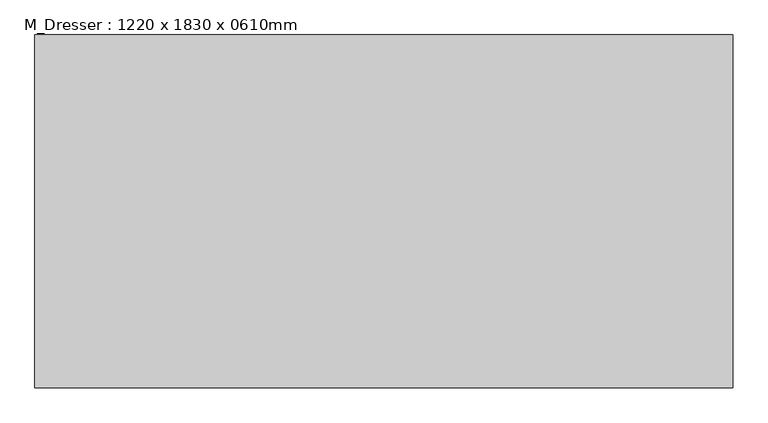
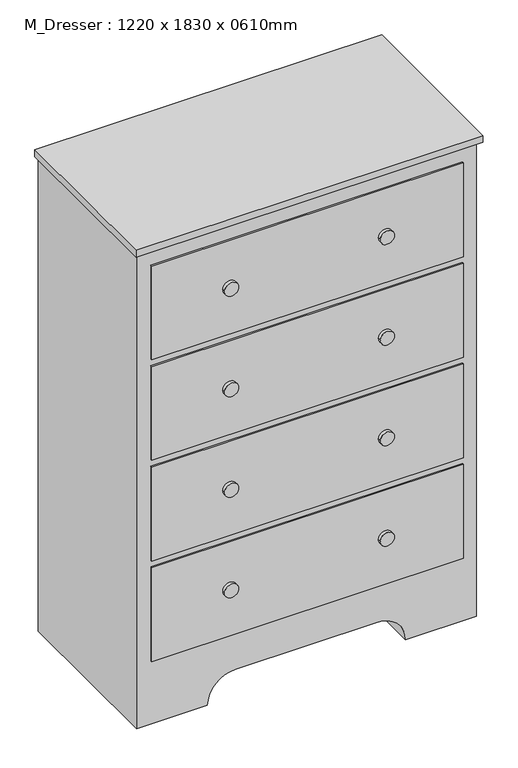
"""IFC4 building model written with IfcOpenShell, lengths in millimetres: furniture geometry, M_Dresser : 1220 x 1830 x 0610mm."""

from ifc_helpers import new_model, si_unit, point, frame, frame_2d, origin, place, context, project, spatial, polyline, circle_curve, trimmed, segment, composite_curve, outline, extrude, source, transform, mapped, element, save


def m_dresser_1220_x_1830_x_0610mm_75a9f440(model_context):
    return source(origin(), model_context, "Body", "SweptSolid", [
        extrude(outline(composite_curve([segment(polyline([(0.0, 340.8067402), (1804.6, 340.8067402), (1804.6, -879.1932598), (0.0, -879.1932598), (0.0, -625.1932598)]), True, "CONTINUOUS"), segment(trimmed(circle_curve(frame_2d((0.0, -523.5932598)), 101.6), [point((0.0, -625.1932598))], [point((101.6, -523.5932598))], True, "CARTESIAN"), True, "CONTINUOUS"), segment(polyline([(101.6, -523.5932598), (101.6, -14.7932598)]), True, "CONTINUOUS"), segment(trimmed(circle_curve(frame_2d((0.0, -14.7932598)), 101.6), [point((101.6, -14.7932598))], [point((0.0, 86.8067402))], True, "CARTESIAN"), True, "CONTINUOUS"), segment(polyline([(0.0, 86.8067402), (0.0, 340.8067402)]), True, "CONTINUOUS")], self_intersect=False)), frame((0.0, -668.1629541, 0.0), z_axis=(0.0, 1.0, 0.0), x_axis=(0.0, 0.0, 1.0)), (0.0, 0.0, 1.0), 610.0),
        extrude(outline(polyline([(353.5067402, -58.1629541), (353.5067402, -687.2129541), (-891.8932598, -687.2129541), (-891.8932598, -58.1629541), (353.5067402, -58.1629541)])), frame((0.0, 0.0, 1804.6), z_axis=(0.0, 0.0, 1.0), x_axis=(1.0, 0.0, 0.0)), (0.0, 0.0, 1.0), 25.4),
        extrude(outline(polyline([(290.0067402, -674.5129541), (-828.3932598, -674.5129541), (-828.3932598, -668.1629541), (290.0067402, -668.1629541), (290.0067402, -674.5129541)])), frame((0.0, 0.0, 1385.2), z_axis=(0.0, 0.0, 1.0), x_axis=(1.0, 0.0, 0.0)), (0.0, 0.0, 1.0), 355.9),
        extrude(outline(polyline([(290.0067402, -674.5129541), (-828.3932598, -674.5129541), (-828.3932598, -668.1629541), (290.0067402, -668.1629541), (290.0067402, -674.5129541)])), frame((0.0, 0.0, 1003.9), z_axis=(0.0, 0.0, 1.0), x_axis=(1.0, 0.0, 0.0)), (0.0, 0.0, 1.0), 355.9),
        extrude(outline(polyline([(290.0067402, -674.5129541), (-828.3932598, -674.5129541), (-828.3932598, -668.1629541), (290.0067402, -668.1629541), (290.0067402, -674.5129541)])), frame((0.0, 0.0, 622.6), z_axis=(0.0, 0.0, 1.0), x_axis=(1.0, 0.0, 0.0)), (0.0, 0.0, 1.0), 355.9),
        extrude(outline(polyline([(290.0067402, -674.5129541), (-828.3932598, -674.5129541), (-828.3932598, -668.1629541), (290.0067402, -668.1629541), (290.0067402, -674.5129541)])), frame((0.0, 0.0, 241.3), z_axis=(0.0, 0.0, 1.0), x_axis=(1.0, 0.0, 0.0)), (0.0, 0.0, 1.0), 355.9),
        extrude(outline(composite_curve([segment(trimmed(circle_curve(frame_2d((1563.15, 10.4067402)), 25.4), [point((1563.15, -14.9932598))], [point((1563.15, 35.8067402))], False, "CARTESIAN"), True, "CONTINUOUS"), segment(trimmed(circle_curve(frame_2d((1563.15, 10.4067402)), 25.4), [point((1563.15, 35.8067402))], [point((1563.15, -14.9932598))], False, "CARTESIAN"), True, "CONTINUOUS")], self_intersect=False)), frame((0.0, -687.2129541, 0.0), z_axis=(0.0, 1.0, 0.0), x_axis=(0.0, 0.0, 1.0)), (0.0, 0.0, 1.0), 12.7),
        extrude(outline(composite_curve([segment(trimmed(circle_curve(frame_2d((1181.85, 10.4067402)), 25.4), [point((1181.85, -14.9932598))], [point((1181.85, 35.8067402))], False, "CARTESIAN"), True, "CONTINUOUS"), segment(trimmed(circle_curve(frame_2d((1181.85, 10.4067402)), 25.4), [point((1181.85, 35.8067402))], [point((1181.85, -14.9932598))], False, "CARTESIAN"), True, "CONTINUOUS")], self_intersect=False)), frame((0.0, -687.2129541, 0.0), z_axis=(0.0, 1.0, 0.0), x_axis=(0.0, 0.0, 1.0)), (0.0, 0.0, 1.0), 12.7),
        extrude(outline(composite_curve([segment(trimmed(circle_curve(frame_2d((800.55, 10.4067402)), 25.4), [point((800.55, -14.9932598))], [point((800.55, 35.8067402))], False, "CARTESIAN"), True, "CONTINUOUS"), segment(trimmed(circle_curve(frame_2d((800.55, 10.4067402)), 25.4), [point((800.55, 35.8067402))], [point((800.55, -14.9932598))], False, "CARTESIAN"), True, "CONTINUOUS")], self_intersect=False)), frame((0.0, -687.2129541, 0.0), z_axis=(0.0, 1.0, 0.0), x_axis=(0.0, 0.0, 1.0)), (0.0, 0.0, 1.0), 12.7),
        extrude(outline(composite_curve([segment(trimmed(circle_curve(frame_2d((419.25, 10.4067402)), 25.4), [point((419.25, -14.9932598))], [point((419.25, 35.8067402))], False, "CARTESIAN"), True, "CONTINUOUS"), segment(trimmed(circle_curve(frame_2d((419.25, 10.4067402)), 25.4), [point((419.25, 35.8067402))], [point((419.25, -14.9932598))], False, "CARTESIAN"), True, "CONTINUOUS")], self_intersect=False)), frame((0.0, -687.2129541, 0.0), z_axis=(0.0, 1.0, 0.0), x_axis=(0.0, 0.0, 1.0)), (0.0, 0.0, 1.0), 12.7),
        extrude(outline(composite_curve([segment(trimmed(circle_curve(frame_2d((419.25, -548.7932598)), 25.4), [point((419.25, -574.1932598))], [point((419.25, -523.3932598))], False, "CARTESIAN"), True, "CONTINUOUS"), segment(trimmed(circle_curve(frame_2d((419.25, -548.7932598)), 25.4), [point((419.25, -523.3932598))], [point((419.25, -574.1932598))], False, "CARTESIAN"), True, "CONTINUOUS")], self_intersect=False)), frame((0.0, -687.2129541, 0.0), z_axis=(0.0, 1.0, 0.0), x_axis=(0.0, 0.0, 1.0)), (0.0, 0.0, 1.0), 12.7),
        extrude(outline(composite_curve([segment(trimmed(circle_curve(frame_2d((800.55, -548.7932598)), 25.4), [point((800.55, -574.1932598))], [point((800.55, -523.3932598))], False, "CARTESIAN"), True, "CONTINUOUS"), segment(trimmed(circle_curve(frame_2d((800.55, -548.7932598)), 25.4), [point((800.55, -523.3932598))], [point((800.55, -574.1932598))], False, "CARTESIAN"), True, "CONTINUOUS")], self_intersect=False)), frame((0.0, -687.2129541, 0.0), z_axis=(0.0, 1.0, 0.0), x_axis=(0.0, 0.0, 1.0)), (0.0, 0.0, 1.0), 12.7),
        extrude(outline(composite_curve([segment(trimmed(circle_curve(frame_2d((1181.85, -548.7932598)), 25.4), [point((1181.85, -574.1932598))], [point((1181.85, -523.3932598))], False, "CARTESIAN"), True, "CONTINUOUS"), segment(trimmed(circle_curve(frame_2d((1181.85, -548.7932598)), 25.4), [point((1181.85, -523.3932598))], [point((1181.85, -574.1932598))], False, "CARTESIAN"), True, "CONTINUOUS")], self_intersect=False)), frame((0.0, -687.2129541, 0.0), z_axis=(0.0, 1.0, 0.0), x_axis=(0.0, 0.0, 1.0)), (0.0, 0.0, 1.0), 12.7),
        extrude(outline(composite_curve([segment(trimmed(circle_curve(frame_2d((1563.15, -548.7932598)), 25.4), [point((1563.15, -574.1932598))], [point((1563.15, -523.3932598))], False, "CARTESIAN"), True, "CONTINUOUS"), segment(trimmed(circle_curve(frame_2d((1563.15, -548.7932598)), 25.4), [point((1563.15, -523.3932598))], [point((1563.15, -574.1932598))], False, "CARTESIAN"), True, "CONTINUOUS")], self_intersect=False)), frame((0.0, -687.2129541, 0.0), z_axis=(0.0, 1.0, 0.0), x_axis=(0.0, 0.0, 1.0)), (0.0, 0.0, 1.0), 12.7),
    ])


if __name__ == "__main__":
    model = new_model("IFC4")
    model_context = context("Model", 3, world=origin())
    ifc_project = project(units=[si_unit("LENGTHUNIT", "METRE", prefix="MILLI")], contexts=[model_context])
    site = spatial("IfcSite", under=ifc_project)
    building = spatial("IfcBuilding", under=site)
    placement = place(None, origin())
    m_dresser_1220_x_1830_x_0610mm_shape = m_dresser_1220_x_1830_x_0610mm_75a9f440(model_context)
    element("IfcFurniture", 1, ObjectType="M_Dresser : 1220 x 1830 x 0610mm", at=placement, inside=building, context=model_context, shape_type="MappedRepresentation", body=[
        mapped(m_dresser_1220_x_1830_x_0610mm_shape, transform((0.0, 0.0, 0.0), x_axis=(1.0, 0.0, 0.0), y_axis=(0.0, 1.0, 0.0), z_axis=(0.0, 0.0, 1.0))),
    ])
    save(model, "model.ifc")

# Revit data of these elements
# Type "M_Dresser : 1220 x 1830 x 0610mm"
#   Depth = 2.001312 ft
#   Height = 6.003937 ft
#   Width = 4.002625 ft
#   Dresser Material = Laminate - Ivory, Glossy
#   Drawer Material = Laminate, Ivory, Matte
#   Knob Material = Cherry
#   Default Elevation = 0
# Element 1 (IfcFurniture, "M_Dresser : 1220 x 1830 x 0610mm")
#   Materials on its faces: "Laminate, Ivory, Matte", "Cherry", "Laminate - Ivory, Glossy"
# Materials
#   "Laminate - Ivory, Glossy": colour RGB 247 247 239, transparency 0
#   "Laminate, Ivory, Matte": class "Plastic", colour RGB 247 247 239, transparency 0, Description = "Plastic Laminate - Ivory, Matte", Cost = 0
#   "Cherry": class "Wood", colour RGB 226 177 128, transparency 0, Description = "Prunus Serotina", Cost = 0
